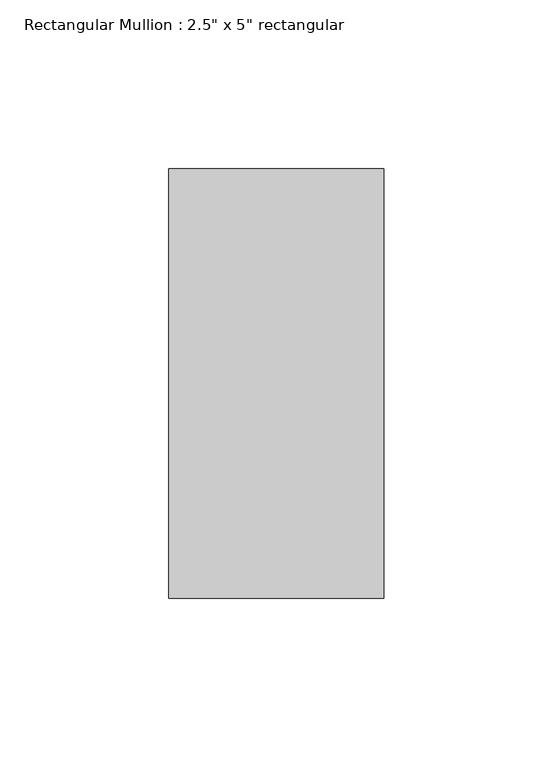
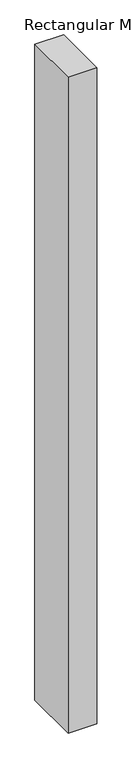
"""IFC4 building model written with IfcOpenShell, lengths in millimetres: member geometry."""

from ifc_helpers import new_model, si_unit, frame, origin, place, context, project, spatial, polyline, outline, extrude, source, transform, mapped, element, save


def member_f2991489(model_context):
    return source(origin(), model_context, "Body", "SweptSolid", [
        extrude(outline(polyline([(31.75, 63.5), (31.75, -63.5), (-31.75, -63.5), (-31.75, 63.5), (31.75, 63.5)])), frame((0.0, 0.0, -1529.3594037), z_axis=(0.0, 0.0, 1.0), x_axis=(1.0, 0.0, 0.0)), (0.0, 0.0, 1.0), 1529.3594037),
    ])


if __name__ == "__main__":
    model = new_model("IFC4")
    model_context = context("Model", 3, world=origin())
    ifc_project = project(units=[si_unit("LENGTHUNIT", "METRE", prefix="MILLI")], contexts=[model_context])
    site = spatial("IfcSite", under=ifc_project)
    building = spatial("IfcBuilding", under=site)
    placement = place(None, origin())
    member_shape = member_f2991489(model_context)
    element("IfcMember", 1, ObjectType="Rectangular Mullion : 2.5\" x 5\" rectangular", at=placement, inside=building, context=model_context, shape_type="MappedRepresentation", body=[
        mapped(member_shape, transform((0.0, 0.0, 0.0), x_axis=(1.0, 0.0, 0.0), y_axis=(0.0, 1.0, 0.0), z_axis=(0.0, 0.0, 1.0))),
    ])
    save(model, "model.ifc")

# Revit data of these elements
# Type "Rectangular Mullion : 2.5\" x 5\" rectangular"
#   built-in parameter 1007304 = 0.416667 (stored number, unit not read)
#   built-in parameter 1007301 = 0.104167 (stored number, unit not read)
#   built-in parameter 1007300 = 0.104167 (stored number, unit not read)
# Element 1 (IfcMember, "Rectangular Mullion : 2.5\" x 5\" rectangular")
#   Materials on its faces: "Aluminum"
# Materials
#   "Aluminum": class "Metal", colour RGB 247 247 247, transparency 0, Description = "Aluminum 6061", Cost = 0
